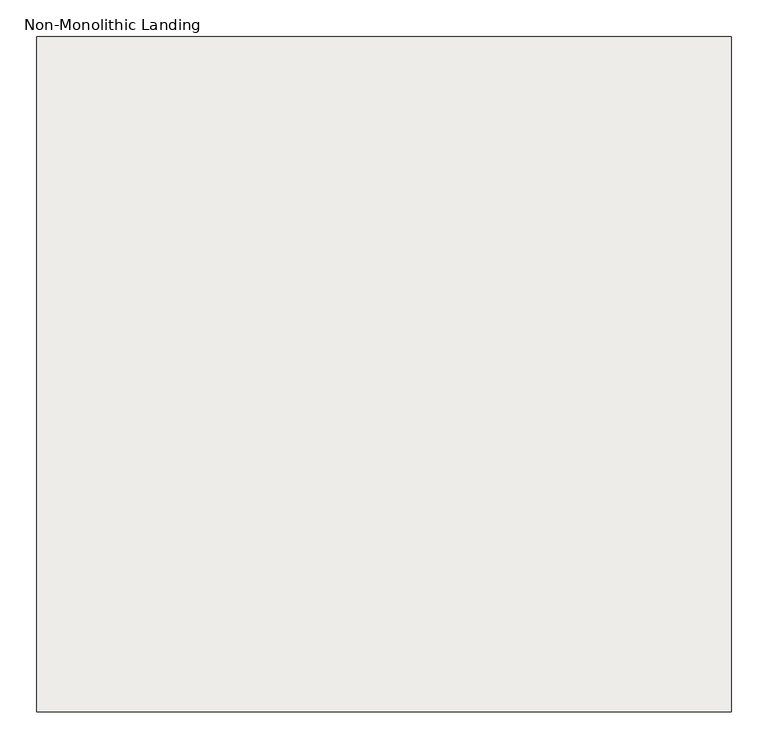
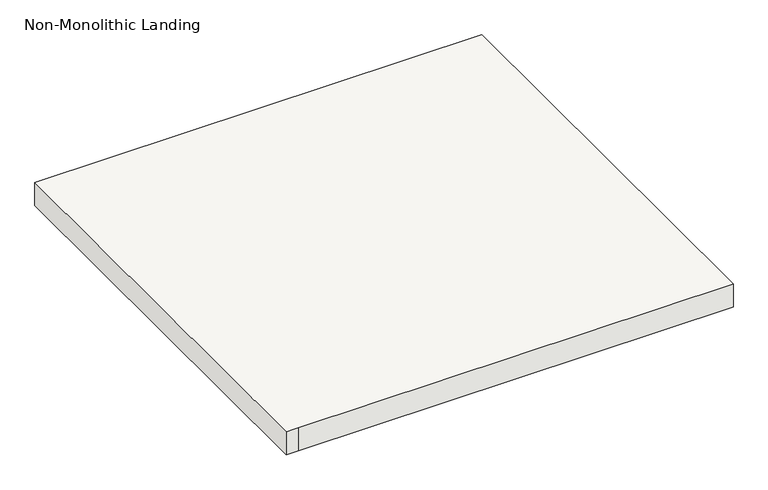
"""IFC4 building model written with IfcOpenShell, lengths in millimetres: slab geometry, Non-Monolithic Landing."""

from ifc_helpers import new_model, si_unit, origin, place, context, project, spatial, faceted_brep, source, transform, mapped, element, save


def non_monolithic_landing_4f0ba0af(model_context):
    return source(origin(), model_context, "Body", "Brep", [
        faceted_brep([(111.2391502, 2117.5115866, 2182.2833333), (111.2391502, 2092.1115866, 2156.8833333), (-803.1608498, 2092.1115866, 2156.8833333), (-803.1608498, 2117.5115866, 2182.2833333), (-828.5608498, 2117.5115866, 2201.3333333), (-828.5608498, 1203.1115866, 2201.3333333), (-803.1608498, 1203.1115866, 2201.3333333), (111.2391502, 1203.1115866, 2201.3333333), (111.2391502, 2117.5115866, 2201.3333333), (-803.1608498, 2092.1115866, 2150.5333333), (111.2391502, 2092.1115866, 2150.5333333), (111.2391502, 1203.1115866, 2150.5333333), (-803.1608498, 1203.1115866, 2150.5333333), (-828.5608498, 1203.1115866, 2150.5333333), (-828.5608498, 2117.5115866, 2150.5333333), (-803.1608498, 2117.5115866, 2150.5333333)], [[[0, 1, 2, 3]], [[4, 5, 6, 7, 8]], [[9, 10, 11, 12, 13, 14, 15]], [[10, 9, 2, 1]], [[9, 15, 3, 2]], [[4, 8, 0, 3, 15, 14]], [[5, 4, 14, 13]], [[6, 5, 13, 12]], [[7, 6, 12, 11]], [[8, 7, 11, 10, 1, 0]]]),
    ])


if __name__ == "__main__":
    model = new_model("IFC4")
    model_context = context("Model", 3, world=origin())
    ifc_project = project(units=[si_unit("LENGTHUNIT", "METRE", prefix="MILLI")], contexts=[model_context])
    site = spatial("IfcSite", under=ifc_project)
    building = spatial("IfcBuilding", under=site)
    placement = place(None, origin())
    non_monolithic_landing_shape = non_monolithic_landing_4f0ba0af(model_context)
    element("IfcSlab", 1, ObjectType="Non-Monolithic Landing", at=placement, inside=building, context=model_context, shape_type="MappedRepresentation", body=[
        mapped(non_monolithic_landing_shape, transform((0.0, 0.0, 0.0), x_axis=(1.0, 0.0, 0.0), y_axis=(0.0, 1.0, 0.0), z_axis=(0.0, 0.0, 1.0))),
    ])
    save(model, "model.ifc")
